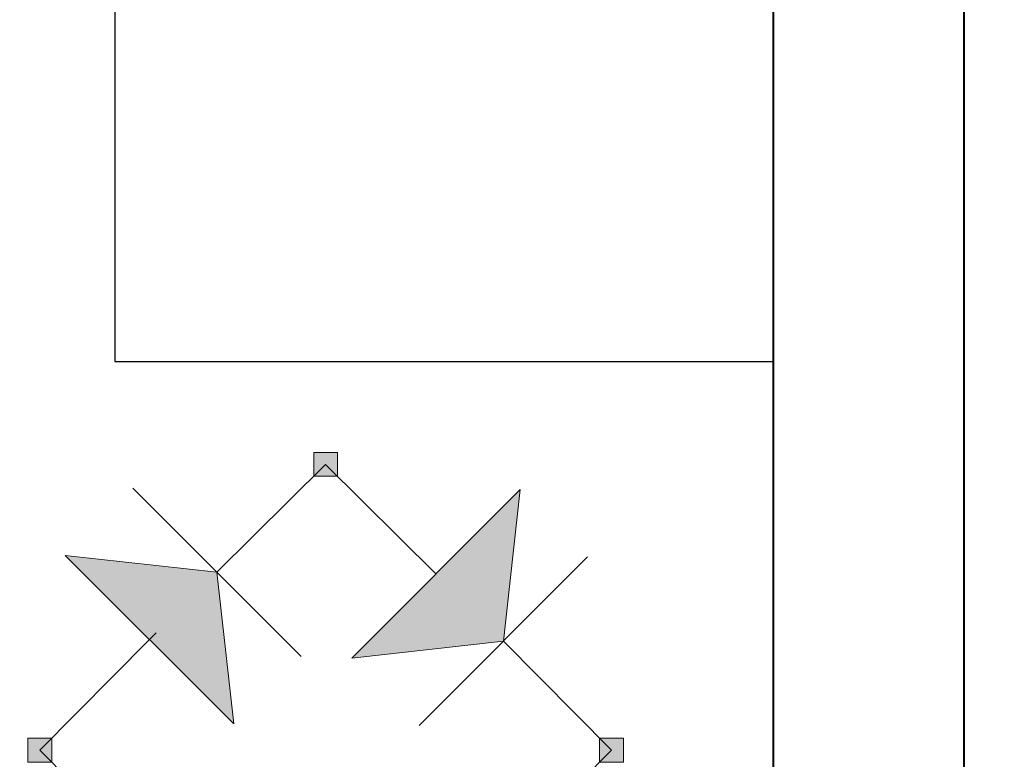
# Model space of a CAD drawing. Units: inches. Extents: x 459864 to 460310, y 324185 to 324787.
# Tile 67 of 112: x 460101 to 460127, y 324302 to 324321. Entities that reach past the tile are written whole.
import ezdxf

# ---------------------------------------------------------------- set-up
doc = ezdxf.new("R2010")
doc.units = ezdxf.units.IN
for name, color, linetype, lineweight in [('A-ANNO-DIMS', 2, 'Continuous', 18), ('A-FLOR-CASE', 8, 'Continuous', 25), ('A-FURN', 8, 'Continuous', 18), ('A-WALL', 7, 'Continuous', 40)]:
    doc.layers.add(name, color=color, linetype=linetype, lineweight=lineweight)
doc.styles.get("Standard").update_dxf_attribs({"font": 'arial.ttf'})
doc.dimstyles.new('ISO-25', dxfattribs={"dimtxt": 6, "dimasz": 2.5, "dimexe": 1.25, "dimexo": 0.625, "dimtad": 1, "dimdec": 1, "dimlunit": 3, "dimtxsty": 'Standard', "dimcen": 2.5, "dimadec": 0, "dimazin": 0, "dimtfac": 1, "dimtdec": 1, "dimtmove": 0, "dimatfit": 3, "dimfxl": 1, "dimarcsym": 0})

# ---------------------------------------------------------------- blocks, each defined once
blk = doc.blocks.new('Full Wave Bridge')
for p, q in [((0.185922, 0.186729), (0.3, 0.3)), ((0.415786, 0.185084), (0.3, 0.3)), ((0.274311, 0.098341), (0.097534, 0.275118)), ((0.327398, 0.096696), (0.504174, 0.273472)), ((0.504174, 0.273472), (0.486497, 0.114373)), ((0.026823, 0.204407), (0.185922, 0.186729)), ((0.2036, 0.02763), (0.026823, 0.204407)), ((0.398109, 0.025985), (0.574885, 0.202762)), ((0.185922, 0.186729), (0.2036, 0.02763)), ((0.115212, 0.116019), (0, 0)), ((0.115212, 0.116019), (0.122283, 0.12309)), ((0.486497, 0.114373), (0.327398, 0.096696)), ((0.486497, 0.114373), (0.6, 0)), ((0.113504, -0.114373), (0, 0)), ((0.486497, -0.114373), (0.6, 0)), ((0.025116, -0.202762), (0.201892, -0.025985)), ((0.574885, -0.202762), (0.398108, -0.025985)), ((0.095826, -0.273472), (0.272603, -0.096695)), ((0.327398, -0.096695), (0.486497, -0.114373)), ((0.504174, -0.273472), (0.327398, -0.096695)), ((0.113504, -0.114373), (0.120575, -0.121444)), ((0.120575, -0.121444), (0.127646, -0.128515)), ((0.486497, -0.114373), (0.504174, -0.273472)), ((0.127646, -0.128515), (0.134717, -0.135586)), ((0.134717, -0.135586), (0.141788, -0.142657)), ((0.141788, -0.142657), (0.15593, -0.1568)), ((0.155993, -0.148218), (0.148824, -0.154349)), ((0.184215, -0.185084), (0.025116, -0.202762)), ((0.184215, -0.185084), (0.3, -0.3)), ((0.415786, -0.185084), (0.3, -0.3)), ((0.415786, -0.185084), (0.422857, -0.178013))]:
    blk.add_line(p, q)
for points in [[(0.2875, 0.2875), (0.2875, 0.3125), (0.3125, 0.3125), (0.3125, 0.2875)], [(-0.0125, -0.0125), (-0.0125, 0.0125), (0.012501, 0.0125), (0.012501, -0.0125)], [(0.5875, -0.0125), (0.5875, 0.0125), (0.6125, 0.0125), (0.6125, -0.0125)], [(0.2875, -0.3125), (0.2875, -0.2875), (0.3125, -0.2875), (0.3125, -0.3125)]]:
    blk.add_lwpolyline(points, close=True)
for points in [[(0.3125, 0.2875), (0.3125, 0.3125), (0.2875, 0.3125)], [(0.2875, 0.3125), (0.2875, 0.2875), (0.3125, 0.2875)], [(0.327398, 0.096696), (0.486497, 0.114373), (0.504174, 0.273472)], [(0.2036, 0.02763), (0.185922, 0.186729), (0.026823, 0.204407)], [(0.012501, -0.0125), (0.012501, 0.0125), (-0.0125, 0.0125)], [(-0.0125, 0.0125), (-0.0125, -0.0125), (0.012501, -0.0125)], [(0.6125, -0.0125), (0.6125, 0.0125), (0.5875, 0.0125)], [(0.5875, 0.0125), (0.5875, -0.0125), (0.6125, -0.0125)], [(0.025116, -0.202762), (0.184215, -0.185084), (0.201892, -0.025985)], [(0.327398, -0.096695), (0.486497, -0.114373), (0.504174, -0.273472)], [(0.3125, -0.3125), (0.3125, -0.2875), (0.2875, -0.2875)], [(0.2875, -0.2875), (0.2875, -0.3125), (0.3125, -0.3125)]]:
    blk.add_solid(points)
blk = doc.blocks.new('*D28')
at = {"layer": 'A-ANNO-DIMS', "color": 0, "lineweight": -2, "transparency": 16777216}
for p, q in [((460148.65, 324370.7), (460136.025, 324370.7)), ((460137.275, 324368.2), (460137.275, 324293.2)), ((460148.65, 324290.7), (460136.025, 324290.7)), ((460137.275, 324290.7), (460137.275, 324198.69))]:
    blk.add_line(p, q, dxfattribs=at)
at = {"layer": 'A-ANNO-DIMS', "color": 0, "transparency": 16777216}
for points in [[(460136.858, 324368.2), (460137.692, 324368.2), (460137.275, 324370.7)], [(460136.858, 324293.2), (460137.692, 324293.2), (460137.275, 324290.7)]]:
    blk.add_solid(points, dxfattribs=at)
at = {"layer": 'Defpoints', "color": 0, "transparency": 16777216}
for p in [(460149.275, 324370.7), (460137.275, 324290.7), (460149.275, 324290.7)]:
    blk.add_point(p, dxfattribs=at)
at = {"layer": 'A-ANNO-DIMS', "color": 0, "transparency": 16777216, "insert": (460133.363, 324243.445), "char_height": 6, "attachment_point": 5, "rotation": 90}
blk.add_mtext('QUEEN BED 6\'-8" TYP.', dxfattribs=at)
blk = doc.blocks.new('*D73')
at = {"layer": 'A-ANNO-DIMS', "color": 0, "lineweight": -2, "transparency": 16777216}
for p, q in [((460109.617, 324339.904), (460082.316, 324311.465)), ((460063.615, 324291.983), (460080.585, 324309.661))]:
    blk.add_line(p, q, dxfattribs=at)
at = {"layer": 'A-ANNO-DIMS', "color": 0, "transparency": 16777216}
blk.add_solid([(460082.016, 324311.753), (460082.617, 324311.176), (460080.585, 324309.661)], dxfattribs=at)
at = {"layer": 'Defpoints', "color": 0, "transparency": 16777216}
for p in [(460080.585, 324309.661), (460063.615, 324291.983)]:
    blk.add_point(p, dxfattribs=at)
at = {"layer": 'A-ANNO-DIMS', "color": 0, "transparency": 16777216, "insert": (460094.144, 324329.167), "char_height": 6, "attachment_point": 5, "rotation": 46.1701}
blk.add_mtext('R2\'-0 1/2"', dxfattribs=at)

msp = doc.modelspace()

# ---------------------------------------------------------------- linework, layer by layer
at = {"layer": 'A-FLOR-CASE'}
for p, q in [((460103.847, 324359.05), (460103.847, 324311.967)), ((460103.847, 324311.967), (460121.115, 324311.967))]:
    msp.add_line(p, q, dxfattribs=at)
at = {"layer": 'A-WALL'}
for p, q in [((460121.115, 324399.05), (460121.115, 324283.483)), ((460126.115, 324399.05), (460126.115, 324283.483))]:
    msp.add_line(p, q, dxfattribs=at)

# ---------------------------------------------------------------- block references
at = {"layer": 'A-FURN', "xscale": 25, "yscale": 25}
msp.add_blockref('Full Wave Bridge', (460101.877, 324301.769), dxfattribs=at)

# ---------------------------------------------------------------- dimensions: what is measured, and where the dimension line sits
at = {"layer": 'A-ANNO-DIMS'}
dim = msp.add_linear_dim(base=(460137.275, 324290.7), p1=(460149.275, 324370.7), p2=(460149.275, 324290.7), angle=270, text='QUEEN BED <> TYP.', dimstyle='ISO-25', override={"dimdec": 1, "dimlfac": 1, "dimrnd": 0, "dimzin": 1, "dimdsep": 46, "dimlunit": 4, "dimfrac": 2}, dxfattribs=at)
dim.commit()
dim.dimension.update_dxf_attribs({"geometry": '*D28', "text_midpoint": (460133.363, 324243.445)})
dim = msp.add_radius_dim(center=(460063.615, 324291.983), mpoint=(460080.585, 324309.661), dimstyle='ISO-25', override={"dimdec": 1, "dimlfac": 1, "dimrnd": 0, "dimzin": 1, "dimdsep": 46, "dimlunit": 4, "dimfrac": 2}, dxfattribs=at)
dim.commit()
dim.dimension.update_dxf_attribs({"geometry": '*D73', "text_midpoint": (460094.144, 324329.167)})

doc.saveas('drawing.dxf')
